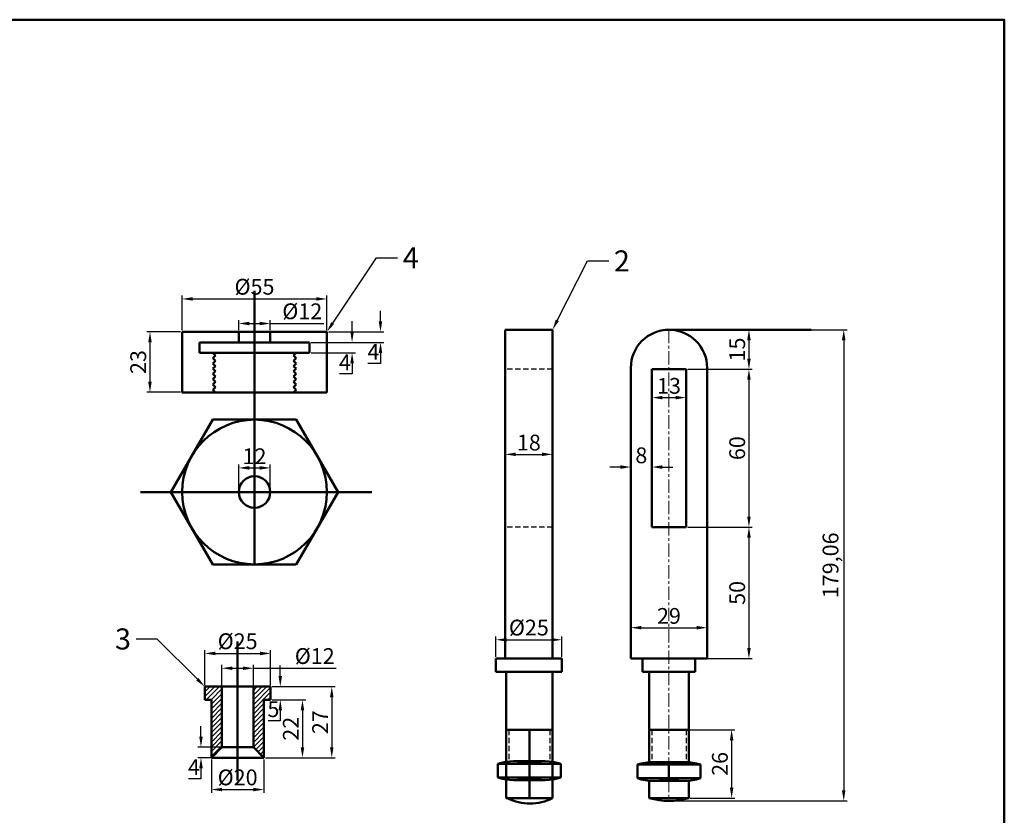
# Model space of a CAD drawing. Units: millimetres. Extents: x -266 to 493, y 251 to 855.
# Tile 3 of 3: x 118 to 493, y 553 to 855. Entities that reach past the tile are written whole.
import ezdxf
from ezdxf import colors
from ezdxf.entities.mleader import LeaderData, LeaderLine
from ezdxf.math import Vec2, Vec3

# ---------------------------------------------------------------- set-up
doc = ezdxf.new("R2010")
doc.units = ezdxf.units.MM
doc.header["$LTSCALE"] = 0.4
doc.linetypes.add('CENTER', pattern=[50.8, 31.75, -6.35, 6.35, -6.35])
doc.linetypes.add('DASHED', pattern=[19.05, 12.7, -6.35])
for name, color, linetype, lineweight in [('M-CNTR', 1, 'CENTER', 18), ('M-DIMS', 2, 'Continuous', 25), ('M-HATC', 8, 'Continuous', 18), ('M-HIDN', 3, 'DASHED', 25), ('M-OUTL', 7, 'Continuous', 50), ('M-TEXT', 7, 'Continuous', 25)]:
    doc.layers.add(name, color=color, linetype=linetype, lineweight=lineweight)
doc.styles.get("Standard").update_dxf_attribs({"font": 'arial.ttf'})
doc.dimstyles.new('ISO-25', dxfattribs={"dimtxt": 6, "dimasz": 4, "dimexe": 1.25, "dimexo": 0.625, "dimtad": 1, "dimtoh": 1, "dimtxsty": 'Standard', "dimcen": 2.5, "dimadec": 0, "dimazin": 0, "dimtfac": 1, "dimtofl": 0, "dimtmove": 0, "dimatfit": 3, "dimfxl": 1, "dimarcsym": 0})

# ---------------------------------------------------------------- blocks, each defined once
blk = doc.blocks.new('*D27')
at = {"layer": 'Defpoints', "color": 0, "transparency": 16777216}
for p in [(213.6, 614.13), (188.6, 601.51), (213.6, 601.51)]:
    blk.add_point(p, dxfattribs=at)
at = {"layer": 'M-DIMS', "color": 0, "lineweight": -2, "transparency": 16777216}
for p, q in [((188.6, 602.13), (188.6, 615.38)), ((192.6, 614.13), (209.6, 614.13)), ((213.6, 602.13), (213.6, 615.38))]:
    blk.add_line(p, q, dxfattribs=at)
at = {"layer": 'M-DIMS', "color": 0, "transparency": 16777216}
for points in [[(192.6, 614.8), (192.6, 613.46), (188.6, 614.13)], [(209.6, 614.8), (209.6, 613.46), (213.6, 614.13)]]:
    blk.add_solid(points, dxfattribs=at)
at = {"layer": 'M-DIMS', "color": 0, "transparency": 16777216, "insert": (201.1, 617.99), "char_height": 6, "attachment_point": 5}
blk.add_mtext('%%C25', dxfattribs=at)
blk = doc.blocks.new('*D28')
at = {"layer": 'Defpoints', "color": 0, "transparency": 16777216}
for p in [(207.1, 608.51), (195.1, 601.51), (207.1, 601.51)]:
    blk.add_point(p, dxfattribs=at)
at = {"layer": 'M-DIMS', "color": 0, "lineweight": -2, "transparency": 16777216}
for p, q in [((195.1, 602.13), (195.1, 609.76)), ((199.1, 608.51), (203.1, 608.51)), ((207.1, 602.13), (207.1, 609.76)), ((207.1, 608.51), (238.55, 608.51))]:
    blk.add_line(p, q, dxfattribs=at)
at = {"layer": 'M-DIMS', "color": 0, "transparency": 16777216}
for points in [[(199.1, 609.17), (199.1, 607.84), (195.1, 608.51)], [(203.1, 609.17), (203.1, 607.84), (207.1, 608.51)]]:
    blk.add_solid(points, dxfattribs=at)
at = {"layer": 'M-DIMS', "color": 0, "transparency": 16777216, "insert": (230.4, 612.36), "char_height": 6, "attachment_point": 5}
blk.add_mtext('%%C12', dxfattribs=at)
blk = doc.blocks.new('*D29')
at = {"layer": 'Defpoints', "color": 0, "transparency": 16777216}
for p in [(201.1, 578.51), (187.16, 574.51), (201.1, 574.51)]:
    blk.add_point(p, dxfattribs=at)
at = {"layer": 'M-DIMS', "color": 0, "lineweight": -2, "transparency": 16777216}
for p, q in [((187.16, 582.51), (187.16, 586.51)), ((200.48, 578.51), (185.91, 578.51)), ((200.48, 574.51), (185.91, 574.51)), ((187.16, 570.51), (187.16, 566.51)), ((187.16, 566.51), (182.38, 566.51))]:
    blk.add_line(p, q, dxfattribs=at)
at = {"layer": 'M-DIMS', "color": 0, "transparency": 16777216}
for points in [[(186.49, 582.51), (187.83, 582.51), (187.16, 578.51)], [(186.49, 570.51), (187.83, 570.51), (187.16, 574.51)]]:
    blk.add_solid(points, dxfattribs=at)
at = {"layer": 'M-DIMS', "color": 0, "transparency": 16777216, "insert": (184.46, 570.13), "char_height": 6, "attachment_point": 5}
blk.add_mtext('4', dxfattribs=at)
blk = doc.blocks.new('*D30')
at = {"layer": 'Defpoints', "color": 0, "transparency": 16777216}
for p in [(191.1, 574.51), (211.1, 574.51), (211.1, 562.4)]:
    blk.add_point(p, dxfattribs=at)
at = {"layer": 'M-DIMS', "color": 0, "lineweight": -2, "transparency": 16777216}
for p, q in [((191.1, 573.88), (191.1, 561.15)), ((211.1, 573.88), (211.1, 561.15)), ((195.1, 562.4), (207.1, 562.4))]:
    blk.add_line(p, q, dxfattribs=at)
at = {"layer": 'M-DIMS', "color": 0, "transparency": 16777216}
for points in [[(195.1, 563.06), (195.1, 561.73), (191.1, 562.4)], [(207.1, 563.06), (207.1, 561.73), (211.1, 562.4)]]:
    blk.add_solid(points, dxfattribs=at)
at = {"layer": 'M-DIMS', "color": 0, "transparency": 16777216, "insert": (201.1, 566.25), "char_height": 6, "attachment_point": 5}
blk.add_mtext('%%C20', dxfattribs=at)
blk = doc.blocks.new('*D31')
at = {"layer": 'Defpoints', "color": 0, "transparency": 16777216}
for p in [(213.6, 601.51), (213.6, 596.51), (217.3, 596.51)]:
    blk.add_point(p, dxfattribs=at)
at = {"layer": 'M-DIMS', "color": 0, "lineweight": -2, "transparency": 16777216}
for p, q in [((217.3, 605.51), (217.3, 609.51)), ((214.23, 601.51), (218.55, 601.51)), ((214.23, 596.51), (218.55, 596.51)), ((217.3, 592.51), (217.3, 588.51)), ((217.3, 588.51), (212.7, 588.51))]:
    blk.add_line(p, q, dxfattribs=at)
at = {"layer": 'M-DIMS', "color": 0, "transparency": 16777216}
for points in [[(216.64, 605.51), (217.97, 605.51), (217.3, 601.51)], [(216.64, 592.51), (217.97, 592.51), (217.3, 596.51)]]:
    blk.add_solid(points, dxfattribs=at)
at = {"layer": 'M-DIMS', "color": 0, "transparency": 16777216, "insert": (214.69, 592.18), "char_height": 6, "attachment_point": 5}
blk.add_mtext('5', dxfattribs=at)
blk = doc.blocks.new('*D32')
at = {"layer": 'Defpoints', "color": 0, "transparency": 16777216}
for p in [(213.6, 596.51), (211.1, 574.51), (225.74, 574.51)]:
    blk.add_point(p, dxfattribs=at)
at = {"layer": 'M-DIMS', "color": 0, "lineweight": -2, "transparency": 16777216}
for p, q in [((214.23, 596.51), (226.99, 596.51)), ((225.74, 592.51), (225.74, 578.51)), ((211.73, 574.51), (226.99, 574.51))]:
    blk.add_line(p, q, dxfattribs=at)
at = {"layer": 'M-DIMS', "color": 0, "transparency": 16777216}
for points in [[(225.07, 592.51), (226.41, 592.51), (225.74, 596.51)], [(225.07, 578.51), (226.41, 578.51), (225.74, 574.51)]]:
    blk.add_solid(points, dxfattribs=at)
at = {"layer": 'M-DIMS', "color": 0, "transparency": 16777216, "insert": (222.1, 585.51), "char_height": 6, "attachment_point": 5, "rotation": 90}
blk.add_mtext('22', dxfattribs=at)
blk = doc.blocks.new('*D33')
at = {"layer": 'Defpoints', "color": 0, "transparency": 16777216}
for p in [(213.6, 601.51), (211.1, 574.51), (236.87, 574.51)]:
    blk.add_point(p, dxfattribs=at)
at = {"layer": 'M-DIMS', "color": 0, "lineweight": -2, "transparency": 16777216}
for p, q in [((214.23, 601.51), (238.12, 601.51)), ((236.87, 597.51), (236.87, 578.51)), ((211.73, 574.51), (238.12, 574.51))]:
    blk.add_line(p, q, dxfattribs=at)
at = {"layer": 'M-DIMS', "color": 0, "transparency": 16777216}
for points in [[(236.2, 597.51), (237.53, 597.51), (236.87, 601.51)], [(236.2, 578.51), (237.53, 578.51), (236.87, 574.51)]]:
    blk.add_solid(points, dxfattribs=at)
at = {"layer": 'M-DIMS', "color": 0, "transparency": 16777216, "insert": (233.23, 588.01), "char_height": 6, "attachment_point": 5, "rotation": 90}
blk.add_mtext('27', dxfattribs=at)
blk = doc.blocks.new('*D53')
at = {"layer": 'Defpoints', "color": 0, "transparency": 16777216}
for p in [(235, 748.86), (180, 736.37), (235, 736.37)]:
    blk.add_point(p, dxfattribs=at)
at = {"layer": 'M-DIMS', "color": 0, "lineweight": -2, "transparency": 16777216}
for p, q in [((180, 736.99), (180, 750.11)), ((184, 748.86), (231, 748.86)), ((235, 736.99), (235, 750.11))]:
    blk.add_line(p, q, dxfattribs=at)
at = {"layer": 'M-DIMS', "color": 0, "transparency": 16777216}
for points in [[(184, 749.53), (184, 748.2), (180, 748.86)], [(231, 749.53), (231, 748.2), (235, 748.86)]]:
    blk.add_solid(points, dxfattribs=at)
at = {"layer": 'M-DIMS', "color": 0, "transparency": 16777216, "insert": (207.5, 752.72), "char_height": 6, "attachment_point": 5}
blk.add_mtext('%%C55', dxfattribs=at)
blk = doc.blocks.new('*D54')
at = {"layer": 'Defpoints', "color": 0, "transparency": 16777216}
for p in [(213.5, 739.53), (201.5, 736.37), (213.5, 736.37)]:
    blk.add_point(p, dxfattribs=at)
at = {"layer": 'M-DIMS', "color": 0, "lineweight": -2, "transparency": 16777216}
for p, q in [((201.5, 736.99), (201.5, 740.78)), ((205.5, 739.53), (209.5, 739.53)), ((213.5, 736.99), (213.5, 740.78)), ((213.5, 739.53), (233.82, 739.53))]:
    blk.add_line(p, q, dxfattribs=at)
at = {"layer": 'M-DIMS', "color": 0, "transparency": 16777216}
for points in [[(205.5, 740.2), (205.5, 738.87), (201.5, 739.53)], [(209.5, 740.2), (209.5, 738.87), (213.5, 739.53)]]:
    blk.add_solid(points, dxfattribs=at)
at = {"layer": 'M-DIMS', "color": 0, "transparency": 16777216, "insert": (225.66, 743.39), "char_height": 6, "attachment_point": 5}
blk.add_mtext('%%C12', dxfattribs=at)
blk = doc.blocks.new('*D55')
at = {"layer": 'Defpoints', "color": 0, "transparency": 16777216}
for p in [(180, 736.37), (167.77, 713.37), (180, 713.37)]:
    blk.add_point(p, dxfattribs=at)
at = {"layer": 'M-DIMS', "color": 0, "lineweight": -2, "transparency": 16777216}
for p, q in [((179.38, 736.37), (166.52, 736.37)), ((167.77, 732.37), (167.77, 717.37)), ((179.38, 713.37), (166.52, 713.37))]:
    blk.add_line(p, q, dxfattribs=at)
at = {"layer": 'M-DIMS', "color": 0, "transparency": 16777216}
for points in [[(167.1, 732.37), (168.43, 732.37), (167.77, 736.37)], [(167.1, 717.37), (168.43, 717.37), (167.77, 713.37)]]:
    blk.add_solid(points, dxfattribs=at)
at = {"layer": 'M-DIMS', "color": 0, "transparency": 16777216, "insert": (164.08, 724.87), "char_height": 6, "attachment_point": 5, "rotation": 90}
blk.add_mtext('23', dxfattribs=at)
blk = doc.blocks.new('*D56')
at = {"layer": 'Defpoints', "color": 0, "transparency": 16777216}
for p in [(235, 736.37), (228.38, 732.37), (255.39, 732.37)]:
    blk.add_point(p, dxfattribs=at)
at = {"layer": 'M-DIMS', "color": 0, "lineweight": -2, "transparency": 16777216}
for p, q in [((255.39, 740.37), (255.39, 744.37)), ((235.63, 736.37), (256.64, 736.37)), ((229.01, 732.37), (256.64, 732.37)), ((255.39, 728.37), (255.39, 724.37)), ((255.39, 724.37), (250.61, 724.37))]:
    blk.add_line(p, q, dxfattribs=at)
at = {"layer": 'M-DIMS', "color": 0, "transparency": 16777216}
for points in [[(254.72, 740.37), (256.05, 740.37), (255.39, 736.37)], [(254.72, 728.37), (256.05, 728.37), (255.39, 732.37)]]:
    blk.add_solid(points, dxfattribs=at)
at = {"layer": 'M-DIMS', "color": 0, "transparency": 16777216, "insert": (252.69, 727.99), "char_height": 6, "attachment_point": 5}
blk.add_mtext('4', dxfattribs=at)
blk = doc.blocks.new('*D57')
at = {"layer": 'Defpoints', "color": 0, "transparency": 16777216}
for p in [(228.38, 732.37), (228.38, 728.37), (244.59, 728.37)]:
    blk.add_point(p, dxfattribs=at)
at = {"layer": 'M-DIMS', "color": 0, "lineweight": -2, "transparency": 16777216}
for p, q in [((244.59, 736.37), (244.59, 740.37)), ((229.01, 732.37), (245.84, 732.37)), ((229.01, 728.37), (245.84, 728.37)), ((244.59, 724.37), (244.59, 720.37)), ((244.59, 720.37), (239.82, 720.37))]:
    blk.add_line(p, q, dxfattribs=at)
at = {"layer": 'M-DIMS', "color": 0, "transparency": 16777216}
for points in [[(243.93, 736.37), (245.26, 736.37), (244.59, 732.37)], [(243.93, 724.37), (245.26, 724.37), (244.59, 728.37)]]:
    blk.add_solid(points, dxfattribs=at)
at = {"layer": 'M-DIMS', "color": 0, "transparency": 16777216, "insert": (241.89, 723.99), "char_height": 6, "attachment_point": 5}
blk.add_mtext('4', dxfattribs=at)
blk = doc.blocks.new('*D58')
at = {"layer": 'Defpoints', "color": 0, "transparency": 16777216}
for p in [(213.5, 684.65), (201.5, 675.49), (213.5, 675.49)]:
    blk.add_point(p, dxfattribs=at)
at = {"layer": 'M-DIMS', "color": 0, "lineweight": -2, "transparency": 16777216}
for p, q in [((201.5, 676.11), (201.5, 685.9)), ((213.5, 676.11), (213.5, 685.9)), ((205.5, 684.65), (209.5, 684.65))]:
    blk.add_line(p, q, dxfattribs=at)
at = {"layer": 'M-DIMS', "color": 0, "transparency": 16777216}
for points in [[(205.5, 685.32), (205.5, 683.99), (201.5, 684.65)], [(209.5, 685.32), (209.5, 683.99), (213.5, 684.65)]]:
    blk.add_solid(points, dxfattribs=at)
at = {"layer": 'M-DIMS', "color": 0, "transparency": 16777216, "insert": (207.5, 688.29), "char_height": 6, "attachment_point": 5}
blk.add_mtext('12', dxfattribs=at)
blk = doc.blocks.new('*D59')
at = {"layer": 'Defpoints', "color": 0, "ltscale": 0.4, "transparency": 16777216}
for p in [(399.28, 737.15), (365.04, 558.1), (431.47, 558.1)]:
    blk.add_point(p, dxfattribs=at)
at = {"layer": 'M-DIMS', "color": 0, "lineweight": -2, "ltscale": 0.4, "transparency": 16777216}
for p, q in [((399.91, 737.15), (432.72, 737.15)), ((431.47, 733.15), (431.47, 562.1)), ((365.66, 558.1), (432.72, 558.1))]:
    blk.add_line(p, q, dxfattribs=at)
at = {"layer": 'M-DIMS', "color": 0, "ltscale": 0.4, "transparency": 16777216}
for points in [[(430.8, 733.15), (432.13, 733.15), (431.47, 737.15)], [(430.8, 562.1), (432.13, 562.1), (431.47, 558.1)]]:
    blk.add_solid(points, dxfattribs=at)
at = {"layer": 'M-DIMS', "color": 0, "ltscale": 0.4, "transparency": 16777216, "insert": (427.23, 647.62), "char_height": 6, "attachment_point": 5, "rotation": 90}
blk.add_mtext('179,06', dxfattribs=at)
blk = doc.blocks.new('*D60')
at = {"layer": 'Defpoints', "color": 0, "ltscale": 0.4, "transparency": 16777216}
for p in [(358.54, 713.85), (371.54, 713.85), (371.54, 711.36)]:
    blk.add_point(p, dxfattribs=at)
at = {"layer": 'M-DIMS', "color": 0, "lineweight": -2, "ltscale": 0.4, "transparency": 16777216}
for p, q in [((358.54, 713.22), (358.54, 710.11)), ((362.54, 711.36), (367.54, 711.36)), ((371.54, 713.22), (371.54, 710.11))]:
    blk.add_line(p, q, dxfattribs=at)
at = {"layer": 'M-DIMS', "color": 0, "ltscale": 0.4, "transparency": 16777216}
for points in [[(362.54, 712.03), (362.54, 710.7), (358.54, 711.36)], [(367.54, 712.03), (367.54, 710.7), (371.54, 711.36)]]:
    blk.add_solid(points, dxfattribs=at)
at = {"layer": 'M-DIMS', "color": 0, "ltscale": 0.4, "transparency": 16777216, "insert": (365.04, 715.05), "char_height": 6, "attachment_point": 5}
blk.add_mtext('13', dxfattribs=at)
blk = doc.blocks.new('*D61')
at = {"layer": 'Defpoints', "color": 0, "ltscale": 0.4, "transparency": 16777216}
for p in [(379.54, 623.92), (350.54, 612.15), (379.54, 612.15)]:
    blk.add_point(p, dxfattribs=at)
at = {"layer": 'M-DIMS', "color": 0, "lineweight": -2, "ltscale": 0.4, "transparency": 16777216}
for p, q in [((350.54, 612.78), (350.54, 625.17)), ((379.54, 612.78), (379.54, 625.17)), ((354.54, 623.92), (375.54, 623.92))]:
    blk.add_line(p, q, dxfattribs=at)
at = {"layer": 'M-DIMS', "color": 0, "ltscale": 0.4, "transparency": 16777216}
for points in [[(354.54, 624.58), (354.54, 623.25), (350.54, 623.92)], [(375.54, 624.58), (375.54, 623.25), (379.54, 623.92)]]:
    blk.add_solid(points, dxfattribs=at)
at = {"layer": 'M-DIMS', "color": 0, "ltscale": 0.4, "transparency": 16777216, "insert": (365.04, 627.61), "char_height": 6, "attachment_point": 5}
blk.add_mtext('29', dxfattribs=at)
blk = doc.blocks.new('*D62')
at = {"layer": 'Defpoints', "color": 0, "ltscale": 0.4, "transparency": 16777216}
for p in [(371.54, 662.15), (365.04, 612.15), (395.44, 612.15)]:
    blk.add_point(p, dxfattribs=at)
at = {"layer": 'M-DIMS', "color": 0, "lineweight": -2, "ltscale": 0.4, "transparency": 16777216}
for p, q in [((372.16, 662.15), (396.69, 662.15)), ((395.44, 658.15), (395.44, 616.15)), ((365.66, 612.15), (396.69, 612.15))]:
    blk.add_line(p, q, dxfattribs=at)
at = {"layer": 'M-DIMS', "color": 0, "ltscale": 0.4, "transparency": 16777216}
for points in [[(394.77, 658.15), (396.11, 658.15), (395.44, 662.15)], [(394.77, 616.15), (396.11, 616.15), (395.44, 612.15)]]:
    blk.add_solid(points, dxfattribs=at)
at = {"layer": 'M-DIMS', "color": 0, "ltscale": 0.4, "transparency": 16777216, "insert": (391.75, 637.15), "char_height": 6, "attachment_point": 5, "rotation": 90}
blk.add_mtext('50', dxfattribs=at)
blk = doc.blocks.new('*D63')
at = {"layer": 'Defpoints', "color": 0, "ltscale": 0.4, "transparency": 16777216}
for p in [(371.54, 722.15), (371.54, 662.15), (395.44, 662.15)]:
    blk.add_point(p, dxfattribs=at)
at = {"layer": 'M-DIMS', "color": 0, "lineweight": -2, "ltscale": 0.4, "transparency": 16777216}
for p, q in [((372.16, 722.15), (396.69, 722.15)), ((395.44, 718.15), (395.44, 666.15)), ((372.16, 662.15), (396.69, 662.15))]:
    blk.add_line(p, q, dxfattribs=at)
at = {"layer": 'M-DIMS', "color": 0, "ltscale": 0.4, "transparency": 16777216}
for points in [[(394.77, 718.15), (396.11, 718.15), (395.44, 722.15)], [(394.77, 666.15), (396.11, 666.15), (395.44, 662.15)]]:
    blk.add_solid(points, dxfattribs=at)
at = {"layer": 'M-DIMS', "color": 0, "ltscale": 0.4, "transparency": 16777216, "insert": (391.75, 692.15), "char_height": 6, "attachment_point": 5, "rotation": 90}
blk.add_mtext('60', dxfattribs=at)
blk = doc.blocks.new('*D64')
at = {"layer": 'Defpoints', "color": 0, "ltscale": 0.4, "transparency": 16777216}
for p in [(387.18, 737.15), (384.43, 722.15), (395.44, 722.15)]:
    blk.add_point(p, dxfattribs=at)
at = {"layer": 'M-DIMS', "color": 0, "lineweight": -2, "ltscale": 0.4, "transparency": 16777216}
for p, q in [((387.81, 737.15), (396.69, 737.15)), ((395.44, 733.15), (395.44, 726.15)), ((385.05, 722.15), (396.69, 722.15))]:
    blk.add_line(p, q, dxfattribs=at)
at = {"layer": 'M-DIMS', "color": 0, "ltscale": 0.4, "transparency": 16777216}
for points in [[(394.77, 733.15), (396.11, 733.15), (395.44, 737.15)], [(394.77, 726.15), (396.11, 726.15), (395.44, 722.15)]]:
    blk.add_solid(points, dxfattribs=at)
at = {"layer": 'M-DIMS', "color": 0, "ltscale": 0.4, "transparency": 16777216, "insert": (391.75, 729.65), "char_height": 6, "attachment_point": 5, "rotation": 90}
blk.add_mtext('15', dxfattribs=at)
blk = doc.blocks.new('*D65')
at = {"layer": 'Defpoints', "color": 0, "ltscale": 0.4, "transparency": 16777216}
for p in [(350.54, 684.97), (358.54, 684.97), (358.54, 684.97)]:
    blk.add_point(p, dxfattribs=at)
at = {"layer": 'M-DIMS', "color": 0, "lineweight": -2, "ltscale": 0.4, "transparency": 16777216}
for p, q in [((346.54, 684.97), (342.54, 684.97)), ((350.54, 685.59), (350.54, 686.22)), ((358.54, 685.59), (358.54, 686.22)), ((362.54, 684.97), (366.54, 684.97))]:
    blk.add_line(p, q, dxfattribs=at)
at = {"layer": 'M-DIMS', "color": 0, "ltscale": 0.4, "transparency": 16777216}
for points in [[(346.54, 685.64), (346.54, 684.3), (350.54, 684.97)], [(362.54, 685.64), (362.54, 684.3), (358.54, 684.97)]]:
    blk.add_solid(points, dxfattribs=at)
at = {"layer": 'M-DIMS', "color": 0, "ltscale": 0.4, "transparency": 16777216, "insert": (354.54, 688.66), "char_height": 6, "attachment_point": 5}
blk.add_mtext('8', dxfattribs=at)
blk = doc.blocks.new('*D66')
at = {"layer": 'Defpoints', "color": 0, "ltscale": 0.4, "transparency": 16777216}
for p in [(372.54, 585.15), (372.54, 559.15), (388.86, 559.15)]:
    blk.add_point(p, dxfattribs=at)
at = {"layer": 'M-DIMS', "color": 0, "lineweight": -2, "ltscale": 0.4, "transparency": 16777216}
for p, q in [((373.16, 585.15), (390.11, 585.15)), ((388.86, 581.15), (388.86, 563.15)), ((373.16, 559.15), (390.11, 559.15))]:
    blk.add_line(p, q, dxfattribs=at)
at = {"layer": 'M-DIMS', "color": 0, "ltscale": 0.4, "transparency": 16777216}
for points in [[(388.2, 581.15), (389.53, 581.15), (388.86, 585.15)], [(388.2, 563.15), (389.53, 563.15), (388.86, 559.15)]]:
    blk.add_solid(points, dxfattribs=at)
at = {"layer": 'M-DIMS', "color": 0, "ltscale": 0.4, "transparency": 16777216, "insert": (385.17, 572.15), "char_height": 6, "attachment_point": 5, "rotation": 90}
blk.add_mtext('26', dxfattribs=at)
blk = doc.blocks.new('*D67')
at = {"layer": 'Defpoints', "color": 0, "ltscale": 0.4, "transparency": 16777216}
for p in [(324.29, 619.33), (299.29, 612.15), (324.29, 612.15)]:
    blk.add_point(p, dxfattribs=at)
at = {"layer": 'M-DIMS', "color": 0, "lineweight": -2, "ltscale": 0.4, "transparency": 16777216}
for p, q in [((299.29, 612.78), (299.29, 620.58)), ((303.29, 619.33), (320.29, 619.33)), ((324.29, 612.78), (324.29, 620.58))]:
    blk.add_line(p, q, dxfattribs=at)
at = {"layer": 'M-DIMS', "color": 0, "ltscale": 0.4, "transparency": 16777216}
for points in [[(303.29, 619.99), (303.29, 618.66), (299.29, 619.33)], [(320.29, 619.99), (320.29, 618.66), (324.29, 619.33)]]:
    blk.add_solid(points, dxfattribs=at)
at = {"layer": 'M-DIMS', "color": 0, "ltscale": 0.4, "transparency": 16777216, "insert": (311.79, 623.18), "char_height": 6, "attachment_point": 5}
blk.add_mtext('%%C25', dxfattribs=at)
blk = doc.blocks.new('*D68')
at = {"layer": 'Defpoints', "color": 0, "ltscale": 0.4, "transparency": 16777216}
for p in [(302.79, 689.8), (320.79, 689.8), (320.79, 689.8)]:
    blk.add_point(p, dxfattribs=at)
at = {"layer": 'M-DIMS', "color": 0, "lineweight": -2, "ltscale": 0.4, "transparency": 16777216}
for p, q in [((302.79, 690.43), (302.79, 691.05)), ((306.79, 689.8), (316.79, 689.8)), ((320.79, 690.43), (320.79, 691.05))]:
    blk.add_line(p, q, dxfattribs=at)
at = {"layer": 'M-DIMS', "color": 0, "ltscale": 0.4, "transparency": 16777216}
for points in [[(306.79, 690.47), (306.79, 689.14), (302.79, 689.8)], [(316.79, 690.47), (316.79, 689.14), (320.79, 689.8)]]:
    blk.add_solid(points, dxfattribs=at)
at = {"layer": 'M-DIMS', "color": 0, "ltscale": 0.4, "transparency": 16777216, "insert": (311.79, 693.49), "char_height": 6, "attachment_point": 5}
blk.add_mtext('18', dxfattribs=at)
blk = doc.blocks.new('HEX-NUT')
at = {"ltscale": 0.4}
for p, q in [((0, 1), (0, 6.16)), ((0, 6.16), (24, 6.16)), ((24, 6.16), (24, 1)), ((24, 1), (0, 1))]:
    blk.add_line(p, q, dxfattribs=at)
for centre, start, end in [((6, -11.34), 71.0754, 108.9246), ((18, -11.34), 71.0754, 108.9246), ((6, 18.5), 251.0754, 288.9246), ((18, 18.5), 251.0754, 288.9246)]:
    blk.add_arc(centre, 18.5, start, end, dxfattribs=at)

msp = doc.modelspace()

# ---------------------------------------------------------------- hatches: boundary and pattern name
at = {"layer": 'M-HATC'}
h = msp.add_hatch(dxfattribs=at)
h.set_pattern_fill('ANSI31', color=256, scale=0.4)
h.set_pattern_definition([(45, (-913.4185, 282.3618), (-0.8980256, 0.8980256), [])])
h.paths.add_polyline_path([(211.104, 596.506), (213.604, 596.506), (213.604, 601.506), (207.104, 601.506), (207.104, 578.506), (211.104, 574.506)])
h.paths.add_polyline_path([(191.104, 574.506), (195.104, 578.506), (195.104, 601.506), (188.604, 601.506), (188.604, 596.506), (191.104, 596.506)])

# ---------------------------------------------------------------- linework, layer by layer
at = {"layer": 'M-CNTR', "ltscale": 0.4}
msp.add_line((365.04, 737.151), (365.04, 559.151), dxfattribs=at)
at = {"layer": 'M-HIDN', "ltscale": 0.4}
for p, q in [((320.785, 722.151), (302.785, 722.151)), ((320.785, 662.151), (302.785, 662.151)), ((304.151, 585.151), (304.151, 572.151)), ((319.785, 585.151), (319.785, 572.151)), ((358.54, 585.151), (358.54, 572.803)), ((371.54, 585.151), (371.54, 572.803)), ((304.151, 566.987), (304.151, 566.076)), ((319.785, 566.987), (319.785, 566.076))]:
    msp.add_line(p, q, dxfattribs=at)
at = {"layer": 'M-OUTL'}
for p, q in [((207.505, 751.958), (207.505, 702.986)), ((180.005, 736.368), (235.005, 736.368)), ((180.005, 713.368), (180.005, 736.368)), ((201.505, 736.368), (201.505, 732.368)), ((213.505, 736.368), (213.505, 732.368)), ((235.005, 736.368), (235.005, 713.368)), ((186.628, 732.368), (228.382, 732.368)), ((186.628, 732.368), (186.628, 728.368)), ((228.382, 732.368), (228.382, 728.368)), ((186.628, 728.368), (228.382, 728.368)), ((191.628, 728.368), (192.628, 727.368)), ((192.628, 727.368), (191.628, 726.368)), ((191.628, 726.368), (192.628, 725.368)), ((223.382, 728.368), (222.382, 727.368)), ((222.382, 727.368), (223.382, 726.368)), ((223.382, 726.368), (222.382, 725.368)), ((192.628, 725.368), (191.628, 724.368)), ((191.628, 724.368), (192.628, 723.368)), ((192.628, 723.368), (191.628, 722.368)), ((191.628, 722.368), (192.628, 721.368)), ((222.382, 725.368), (223.382, 724.368)), ((223.382, 724.368), (222.382, 723.368)), ((222.382, 723.368), (223.382, 722.368)), ((223.382, 722.368), (222.382, 721.368)), ((192.628, 721.368), (191.628, 720.368)), ((191.628, 720.368), (192.628, 719.368)), ((192.628, 719.368), (191.628, 718.368)), ((222.382, 721.368), (223.382, 720.368)), ((223.382, 720.368), (222.382, 719.368)), ((222.382, 719.368), (223.382, 718.368)), ((191.628, 718.368), (192.628, 717.368)), ((192.628, 717.368), (191.628, 716.368)), ((191.628, 716.368), (192.628, 715.368)), ((192.628, 715.368), (191.628, 714.368)), ((223.382, 718.368), (222.382, 717.368)), ((222.382, 717.368), (223.382, 716.368)), ((223.382, 716.368), (222.382, 715.368)), ((222.382, 715.368), (223.382, 714.368)), ((235.005, 713.368), (180.005, 713.368)), ((191.628, 714.368), (192.628, 713.368)), ((223.382, 714.368), (222.382, 713.368)), ((207.505, 702.986), (207.505, 647.986)), ((164.23, 675.486), (252.047, 675.486)), ((201.104, 618.718), (201.104, 565.874)), ((188.604, 601.506), (213.604, 601.506)), ((188.604, 596.506), (188.604, 601.506)), ((195.104, 601.506), (195.104, 578.506)), ((207.104, 601.506), (207.104, 578.506)), ((213.604, 601.506), (213.604, 596.506)), ((191.104, 596.506), (188.604, 596.506)), ((191.104, 596.506), (191.104, 574.506)), ((213.604, 596.506), (211.104, 596.506)), ((211.104, 596.506), (211.104, 574.506)), ((195.104, 578.506), (191.104, 574.506)), ((195.104, 578.506), (207.104, 578.506)), ((207.104, 578.506), (211.104, 574.506)), ((191.104, 574.506), (211.104, 574.506))]:
    msp.add_line(p, q, dxfattribs=at)
at = {"layer": 'M-OUTL', "ltscale": 0.4}
for p, q in [((320.785, 737.151), (302.785, 737.151)), ((302.785, 737.151), (302.785, 612.151)), ((320.785, 737.151), (320.785, 612.151)), ((379.54, 737.151), (365.04, 737.151)), ((379.54, 737.151), (419.03, 737.151)), ((350.54, 722.651), (350.54, 612.151)), ((379.54, 612.151), (379.54, 722.651)), ((358.54, 722.151), (358.54, 662.151)), ((358.54, 722.151), (371.54, 722.151)), ((371.54, 722.151), (371.54, 662.151)), ((358.54, 662.151), (371.54, 662.151)), ((302.785, 612.151), (299.285, 612.151)), ((299.285, 612.151), (299.285, 607.151)), ((302.785, 612.151), (320.785, 612.151)), ((324.285, 612.151), (320.785, 612.151)), ((324.285, 607.151), (324.285, 612.151)), ((350.54, 612.151), (379.54, 612.151)), ((355.04, 612.151), (355.04, 607.151)), ((375.04, 607.151), (375.04, 612.151)), ((299.285, 607.151), (324.285, 607.151)), ((303.151, 607.151), (303.151, 559.151)), ((320.785, 607.151), (320.785, 559.151)), ((355.04, 607.151), (375.04, 607.151)), ((357.54, 607.151), (357.54, 572.803)), ((372.54, 607.151), (372.54, 572.803)), ((320.785, 585.151), (303.151, 585.151)), ((311.968, 585.151), (311.968, 559.151)), ((357.54, 585.151), (372.54, 585.151)), ((305.968, 573.151), (317.968, 573.151)), ((359.04, 572.864), (371.04, 572.864)), ((353.04, 571.864), (377.04, 571.864)), ((353.04, 566.699), (353.04, 571.864)), ((365.04, 571.864), (365.04, 565.699)), ((377.04, 571.864), (377.04, 566.699)), ((317.968, 565.987), (305.968, 565.987)), ((377.04, 566.699), (353.04, 566.699)), ((357.54, 565.76), (357.54, 559.151)), ((371.04, 565.699), (359.04, 565.699)), ((372.54, 565.76), (372.54, 559.151)), ((320.785, 559.151), (303.151, 559.151)), ((357.54, 559.151), (372.54, 559.151))]:
    msp.add_line(p, q, dxfattribs=at)
msp.add_lwpolyline([(-265.707, 854.992), (492.506, 854.992), (492.506, 250.777), (-265.707, 250.777)], close=True, dxfattribs=at)
at = {"layer": 'M-OUTL'}
msp.add_lwpolyline([(223.382, 647.986), (239.259, 675.486), (223.382, 702.986), (191.628, 702.986), (175.751, 675.486), (191.628, 647.986)], close=True, dxfattribs=at)
for radius in [27.5, 6]:
    msp.add_circle((207.505, 675.486), radius, dxfattribs=at)
at = {"layer": 'M-OUTL', "ltscale": 0.4}
for centre, radius, start, end in [((365.04, 722.651), 14.5, 0, 180), ((359.04, 554.364), 18.5, 71.07536, 108.92464), ((371.04, 554.364), 18.5, 71.07536, 108.92464), ((359.04, 584.199), 18.5, 251.07536, 288.92464), ((371.04, 584.199), 18.5, 251.07536, 288.92464), ((312.225, 575.68), 18.614, 242.62012, 297.37988), ((365.04, 585.27), 27.174, 253.9787, 286.0213)]:
    msp.add_arc(centre, radius, start, end, dxfattribs=at)

# ---------------------------------------------------------------- block references
at = {"layer": 'M-OUTL', "rotation": 180}
msp.add_blockref('HEX-NUT', (323.968, 573.151), dxfattribs=at)

# ---------------------------------------------------------------- dimensions: what is measured, and where the dimension line sits
at = {"layer": 'M-DIMS'}
for base, p1, p2, picture, middle in [((235.005, 748.863), (180.005, 736.368), (235.005, 736.368), '*D53', (207.505, 752.719)), ((213.505, 739.534), (201.505, 736.368), (213.505, 736.368), '*D54', (225.661, 743.39))]:
    dim = msp.add_linear_dim(base=base, p1=p1, p2=p2, text='%%C<>', dimstyle='ISO-25', override={"dimclrd": 0, "dimclre": 0, "dimclrt": 0}, dxfattribs=at)
    dim.commit()
    dim.dimension.update_dxf_attribs({"geometry": picture, "text_midpoint": middle})
for base, p1, p2, picture, middle in [((255.388, 732.368), (235.005, 736.368), (228.382, 732.368), '*D56', (252.688, 727.993)), ((244.594, 728.368), (228.382, 732.368), (228.382, 728.368), '*D57', (241.894, 723.993)), ((167.767, 713.368), (180.005, 736.368), (180.005, 713.368), '*D55', (164.077, 724.868))]:
    dim = msp.add_linear_dim(base=base, p1=p1, p2=p2, angle=90, dimstyle='ISO-25', override={"dimclrd": 0, "dimclre": 0, "dimclrt": 0}, dxfattribs=at)
    dim.commit()
    dim.dimension.update_dxf_attribs({"geometry": picture, "text_midpoint": middle})
at = {"layer": 'M-DIMS', "ltscale": 0.4}
for base, p1, p2, picture, middle in [((431.4654, 558.0957), (399.2847, 737.1512), (365.0397, 558.0957), '*D59', (427.2347, 647.6235)), ((395.441, 722.151), (387.183, 737.151), (384.428, 722.151), '*D64', (391.753, 729.651)), ((395.441, 662.151), (371.54, 722.151), (371.54, 662.151), '*D63', (391.753, 692.151)), ((395.441, 612.151), (371.54, 662.151), (365.04, 612.151), '*D62', (391.753, 637.151)), ((388.863, 559.151), (372.54, 585.151), (372.54, 559.151), '*D66', (385.175, 572.151))]:
    dim = msp.add_linear_dim(base=base, p1=p1, p2=p2, angle=90, dimstyle='ISO-25', override={"dimclrd": 0, "dimclre": 0, "dimclrt": 0}, dxfattribs=at)
    dim.commit()
    dim.dimension.update_dxf_attribs({"geometry": picture, "text_midpoint": middle})
for base, p1, p2, picture, middle in [((371.54, 711.363), (358.54, 713.847), (371.54, 713.847), '*D60', (365.04, 715.053)), ((320.785, 689.804), (302.785, 689.804), (320.785, 689.804), '*D68', (311.785, 693.492)), ((358.54, 684.968), (350.54, 684.968), (358.54, 684.968), '*D65', (354.54, 688.657)), ((379.54, 623.918), (350.54, 612.151), (379.54, 612.151), '*D61', (365.04, 627.606))]:
    dim = msp.add_linear_dim(base=base, p1=p1, p2=p2, dimstyle='ISO-25', override={"dimclrd": 0, "dimclre": 0, "dimclrt": 0}, dxfattribs=at)
    dim.commit()
    dim.dimension.update_dxf_attribs({"geometry": picture, "text_midpoint": middle})
at = {"layer": 'M-DIMS'}
dim = msp.add_linear_dim(base=(213.505, 684.652), p1=(201.505, 675.486), p2=(213.505, 675.486), dimstyle='ISO-25', override={"dimclrd": 0, "dimclre": 0, "dimclrt": 0}, dxfattribs=at)
dim.commit()
dim.dimension.update_dxf_attribs({"geometry": '*D58', "text_midpoint": (207.505, 688.29)})
at = {"layer": 'M-DIMS', "ltscale": 0.4}
dim = msp.add_linear_dim(base=(324.285, 619.328), p1=(299.285, 612.151), p2=(324.285, 612.151), text='%%C<>', dimstyle='ISO-25', override={"dimclrd": 0, "dimclre": 0, "dimclrt": 0}, dxfattribs=at)
dim.commit()
dim.dimension.update_dxf_attribs({"geometry": '*D67', "text_midpoint": (311.785, 623.184)})
at = {"layer": 'M-DIMS'}
for base, p1, p2, picture, middle in [((213.604, 614.131), (188.604, 601.506), (213.604, 601.506), '*D27', (201.104, 614.131)), ((207.104, 608.506), (195.104, 601.506), (207.104, 601.506), '*D28', (230.396, 608.506)), ((211.104, 562.397), (191.104, 574.506), (211.104, 574.506), '*D30', (201.104, 562.397))]:
    dim = msp.add_linear_dim(base=base, p1=p1, p2=p2, text='%%C<>', dimstyle='ISO-25', override={"dimclrd": 0, "dimclre": 0, "dimclrt": 0}, dxfattribs=at)
    dim.commit()
    dim.dimension.update_dxf_attribs({"geometry": picture, "text_midpoint": middle, "dimtype": 160})
for base, p1, p2, picture, middle in [((217.305, 596.506), (213.604, 601.506), (213.604, 596.506), '*D31', (214.691, 588.506)), ((236.867, 574.506), (213.604, 601.506), (211.104, 574.506), '*D33', (236.867, 588.006)), ((225.74, 574.506), (213.604, 596.506), (211.104, 574.506), '*D32', (225.74, 585.506)), ((187.158, 574.506), (201.104, 578.506), (201.104, 574.506), '*D29', (184.458, 566.506))]:
    dim = msp.add_linear_dim(base=base, p1=p1, p2=p2, angle=90, dimstyle='ISO-25', override={"dimclrd": 0, "dimclre": 0, "dimclrt": 0}, dxfattribs=at)
    dim.commit()
    dim.dimension.update_dxf_attribs({"geometry": picture, "text_midpoint": middle, "dimtype": 160})

# ---------------------------------------------------------------- leaders
at = {"layer": 'M-TEXT', "ltscale": 0.4}
ml = msp.add_multileader_mtext('Standard', dxfattribs=at)
ml.set_content('4', color=256)
ml.set_leader_properties()
ml.build(insert=Vec2(0, 0))
ctx = ml.context
ctx.base_point, ctx.char_height, ctx.plane_origin = Vec3(261.873, 764.539), 8, Vec3(235.005, 736.368)
notes = []
notes.append((ctx, [(0, (1, 1, 0), (253.873, 764.539), (1, 0), 8, [(0, [(235.005, 736.368)], 0, [])])]))
ctx.mtext.insert, ctx.mtext.flow_direction = Vec3(263.873, 768.539), 5
ml = msp.add_multileader_mtext('Standard', dxfattribs=at)
ml.set_content('2', color=256)
ml.set_leader_properties()
ml.build(insert=Vec2(0, 0))
ctx = ml.context
ctx.base_point, ctx.char_height, ctx.plane_origin = Vec3(342.129, 763.299), 8, Vec3(320.785, 737.151)
notes.append((ctx, [(0, (1, 1, 0), (334.129, 763.299), (1, 0), 8, [(0, [(320.785, 737.151)], 0, [])])]))
ctx.mtext.insert, ctx.mtext.flow_direction = Vec3(344.129, 767.299), 5
ml = msp.add_multileader_mtext('Standard', dxfattribs=at)
ml.set_content('3', color=256)
ml.set_leader_properties()
ml.build(insert=Vec2(0, 0))
ctx = ml.context
ctx.base_point, ctx.char_height, ctx.plane_origin = Vec3(153.307, 619.564), 8, Vec3(188.604, 601.506)
ctx.text_align_type = 2
notes.append((ctx, [(0, (1, 1, 0), (170.546, 619.564), (-1, 0), 8, [(0, [(188.604, 601.506)], 0, [])])]))
ctx.mtext.insert, ctx.mtext.alignment, ctx.mtext.flow_direction = Vec3(160.546, 623.635), 3, 5
for ctx, leaders in notes:
    for number, flags, end, landing, length, lines in leaders:
        leader = LeaderData()
        leader.index, (leader.has_last_leader_line, leader.has_dogleg_vector, leader.attachment_direction) = number, flags
        leader.last_leader_point, leader.dogleg_vector, leader.dogleg_length = Vec3(end), Vec3(landing), length
        for number, points, colour, breaks in lines:
            line = LeaderLine()
            line.index, line.vertices, line.color, line.breaks = number, Vec3.list(points), colors.encode_raw_color(colour), breaks
            leader.lines.append(line)
        ctx.leaders.append(leader)

doc.saveas('drawing.dxf')
